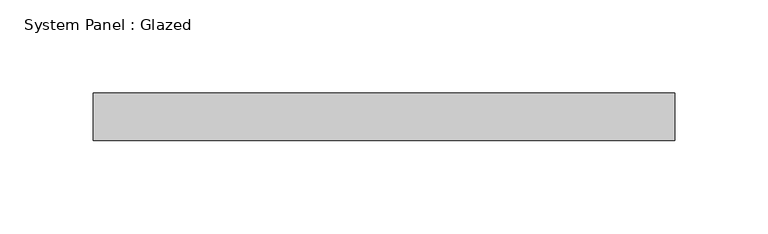
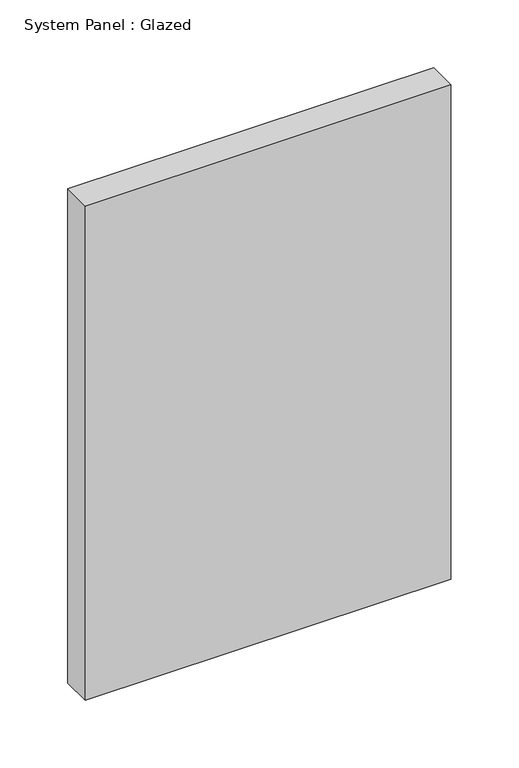
"""IFC4 building model written with IfcOpenShell, lengths in millimetres: plate geometry, System Panel : Glazed."""

from ifc_helpers import new_model, si_unit, origin, origin_with_axes, place, context, project, spatial, polyline, outline, extrude, source, transform, mapped, element, save


def system_panel_glazed_ff0761ce(model_context):
    return source(origin(), model_context, "Body", "SweptSolid", [
        extrude(outline(polyline([(155.575, 19.05), (-155.575, 19.05), (-155.575, 44.45), (155.575, 44.45), (155.575, 19.05)])), origin_with_axes(), (0.0, 0.0, 1.0), 444.5),
    ])


if __name__ == "__main__":
    model = new_model("IFC4")
    model_context = context("Model", 3, world=origin())
    ifc_project = project(units=[si_unit("LENGTHUNIT", "METRE", prefix="MILLI")], contexts=[model_context])
    site = spatial("IfcSite", under=ifc_project)
    building = spatial("IfcBuilding", under=site)
    placement = place(None, origin())
    system_panel_glazed_shape = system_panel_glazed_ff0761ce(model_context)
    element("IfcPlate", 1, ObjectType="System Panel : Glazed", at=placement, inside=building, context=model_context, shape_type="MappedRepresentation", body=[
        mapped(system_panel_glazed_shape, transform((0.0, 0.0, 0.0), x_axis=(1.0, 0.0, 0.0), y_axis=(0.0, 1.0, 0.0), z_axis=(0.0, 0.0, 1.0))),
    ])
    save(model, "model.ifc")

# Revit data of these elements
# Type "System Panel : Glazed"
#   Construction Type Id = "GSP4R"
#   Analytic Construction = "1/8 in Pilkington single glazing"
#   Visual Light Transmittance = 0.9
#   Solar Heat Gain Coefficient = 0.86
#   Heat Transfer Coefficient (U) = 1.18115 BTU/(h·ft²·°F)
#   Define Thermal Properties by = 1
# Element 1 (IfcPlate, "System Panel : Glazed")
#   Materials on its faces: "Glass"
# Materials
#   "Glass": class "Glass", colour RGB 0 128 192, transparency 0.75, Description = "Soda Lime Glass", Cost = 0
